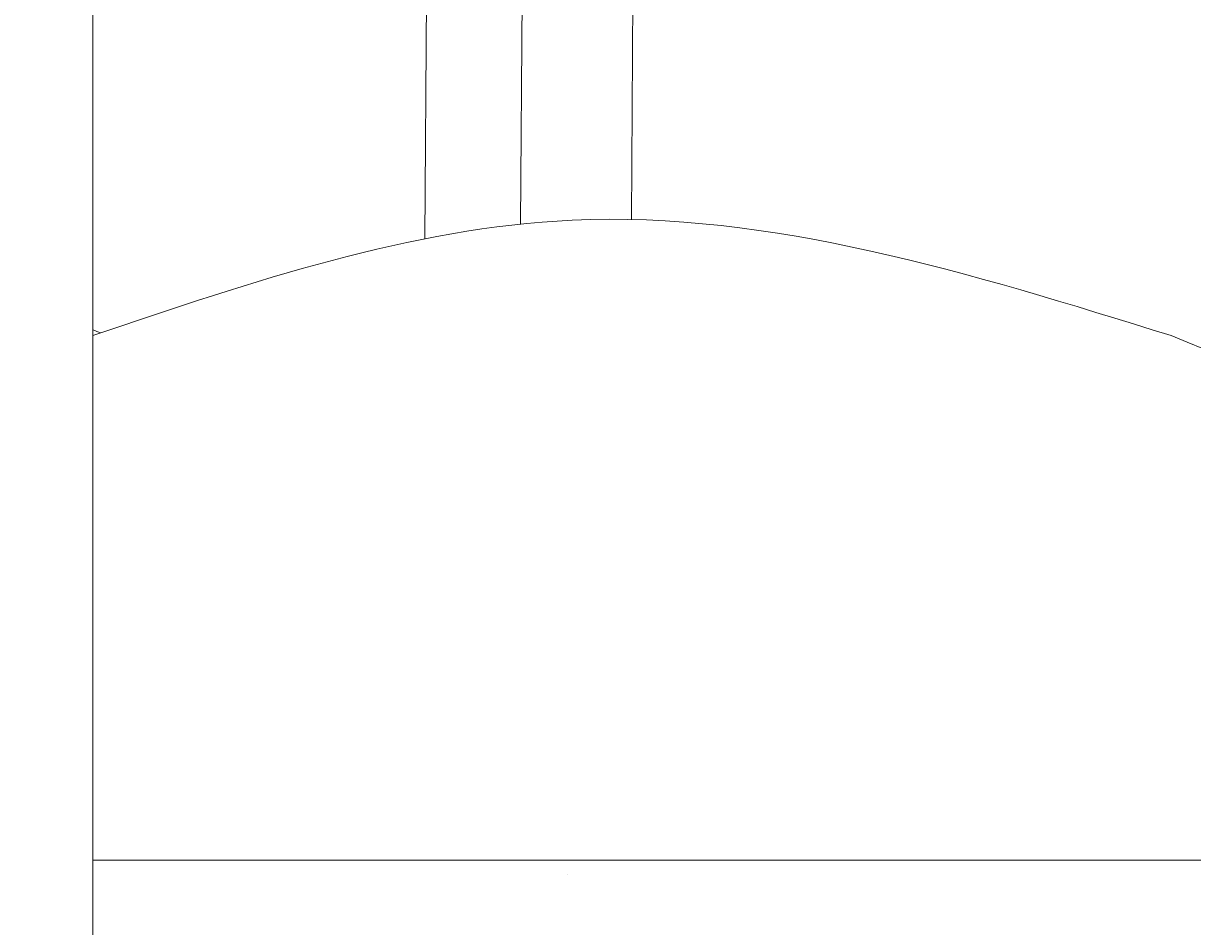
# Model space of a CAD drawing. Units: inches. Extents: x -46 to 1145, y -527 to 760.
# Tile 27 of 57: x 47 to 79, y 252 to 277. Entities that reach past the tile are written whole.
import ezdxf

# ---------------------------------------------------------------- set-up
doc = ezdxf.new("R2010")
doc.units = ezdxf.units.IN
doc.header["$MEASUREMENT"] = 0
doc.layers.add('A-ANNO-DIMS', color=2, linetype='Continuous', lineweight=18)
doc.layers.add('A-FURN', color=2, linetype='Continuous', lineweight=13)
doc.styles.get("Standard").update_dxf_attribs({"font": 'arial.ttf'})
doc.dimstyles.get("Standard").update_dxf_attribs({"dimtxt": 0.18, "dimasz": 0.18, "dimexe": 0.18, "dimexo": 0.0625, "dimgap": 0.09, "dimtad": 0, "dimtih": 1, "dimtoh": 1, "dimdec": 0, "dimzin": 0, "dimdsep": 46, "dimlunit": 3, "dimtxsty": 'Standard', "dimcen": 0.09, "dimadec": 0, "dimazin": 0, "dimtfac": 1, "dimtdec": 0, "dimtofl": 0, "dimtmove": 0, "dimatfit": 3, "dimfxl": 1, "dimtolj": 1, "dimtzin": 0, "dimarcsym": 0})

# ---------------------------------------------------------------- blocks, each defined once
blk = doc.blocks.new('BED-QUEEN-FURNISHED')
for p, q in [((60, 80), (60, 0)), ((46.8, 63.6), (46.799, 63.6)), ((60, 63.2), (0, 63.2)), ((50.463, 0), (50.758, 45.907)), ((44.724, 0), (45.016, 45.372)), ((47.804, 0), (48.097, 45.499))]:
    blk.add_line(p, q)
for centre, radius, start, end in [((15, 13.075), 38.562, 67.1089, 112.8911), ((40.884, -5.132), 56.884, 70.3635, 70.606)]:
    blk.add_arc(centre, radius, start, end)
blk.add_open_spline([(30, 48.601), (35.57, 46.869), (45.642, 43.737), (55.565, 47.098), (60, 48.601)], degree=3, knots=[0, 0, 0, 0, 16.971495, 30.687365, 30.687365, 30.687365, 30.687365])
blk = doc.blocks.new('*D685')
at = {"layer": 'A-ANNO-DIMS', "color": 0, "lineweight": -2, "transparency": 16777216}
for p, q in [((183.501, 700.889), (-46.216, 700.889)), ((-46.036, 700.709), (-46.036, 116.385)), ((-46.036, -468.302), (-46.036, 116.021)), ((12.501, -468.482), (-46.216, -468.482))]:
    blk.add_line(p, q, dxfattribs=at)
at = {"layer": 'A-ANNO-DIMS', "color": 0, "transparency": 16777216}
for points in [[(-46.066, 700.709), (-46.006, 700.709), (-46.036, 700.889)], [(-46.066, -468.302), (-46.006, -468.302), (-46.036, -468.482)]]:
    blk.add_solid(points, dxfattribs=at)
at = {"layer": 'Defpoints', "color": 0, "transparency": 16777216}
for p in [(-46.036, 700.889), (183.564, 700.889), (12.564, -468.482)]:
    blk.add_point(p, dxfattribs=at)
at = {"layer": 'A-ANNO-DIMS', "color": 0, "transparency": 16777216, "insert": (-46.036, 116.203), "char_height": 0.18, "attachment_point": 5}
blk.add_mtext('\\A1;1169.4', dxfattribs=at)

msp = doc.modelspace()

# ---------------------------------------------------------------- block references
at = {"layer": 'A-FURN', "rotation": 180}
msp.add_blockref('BED-QUEEN-FURNISHED', (108.4877, 316.6818), dxfattribs=at)

# ---------------------------------------------------------------- dimensions: what is measured, and where the dimension line sits
at = {"layer": 'A-ANNO-DIMS'}
dim = msp.add_linear_dim(base=(-46.0363, 700.8886), p1=(12.5637, -468.4824), p2=(183.5637, 700.8886), angle=90, dimstyle='Standard', override={"dimdec": 1, "dimlfac": 1, "dimrnd": 0, "dimzin": 0, "dimdsep": 46, "dimlunit": 2}, dxfattribs=at)
dim.commit()
dim.dimension.update_dxf_attribs({"geometry": '*D685', "text_midpoint": (-46.0363, 116.2031)})

doc.saveas('drawing.dxf')
